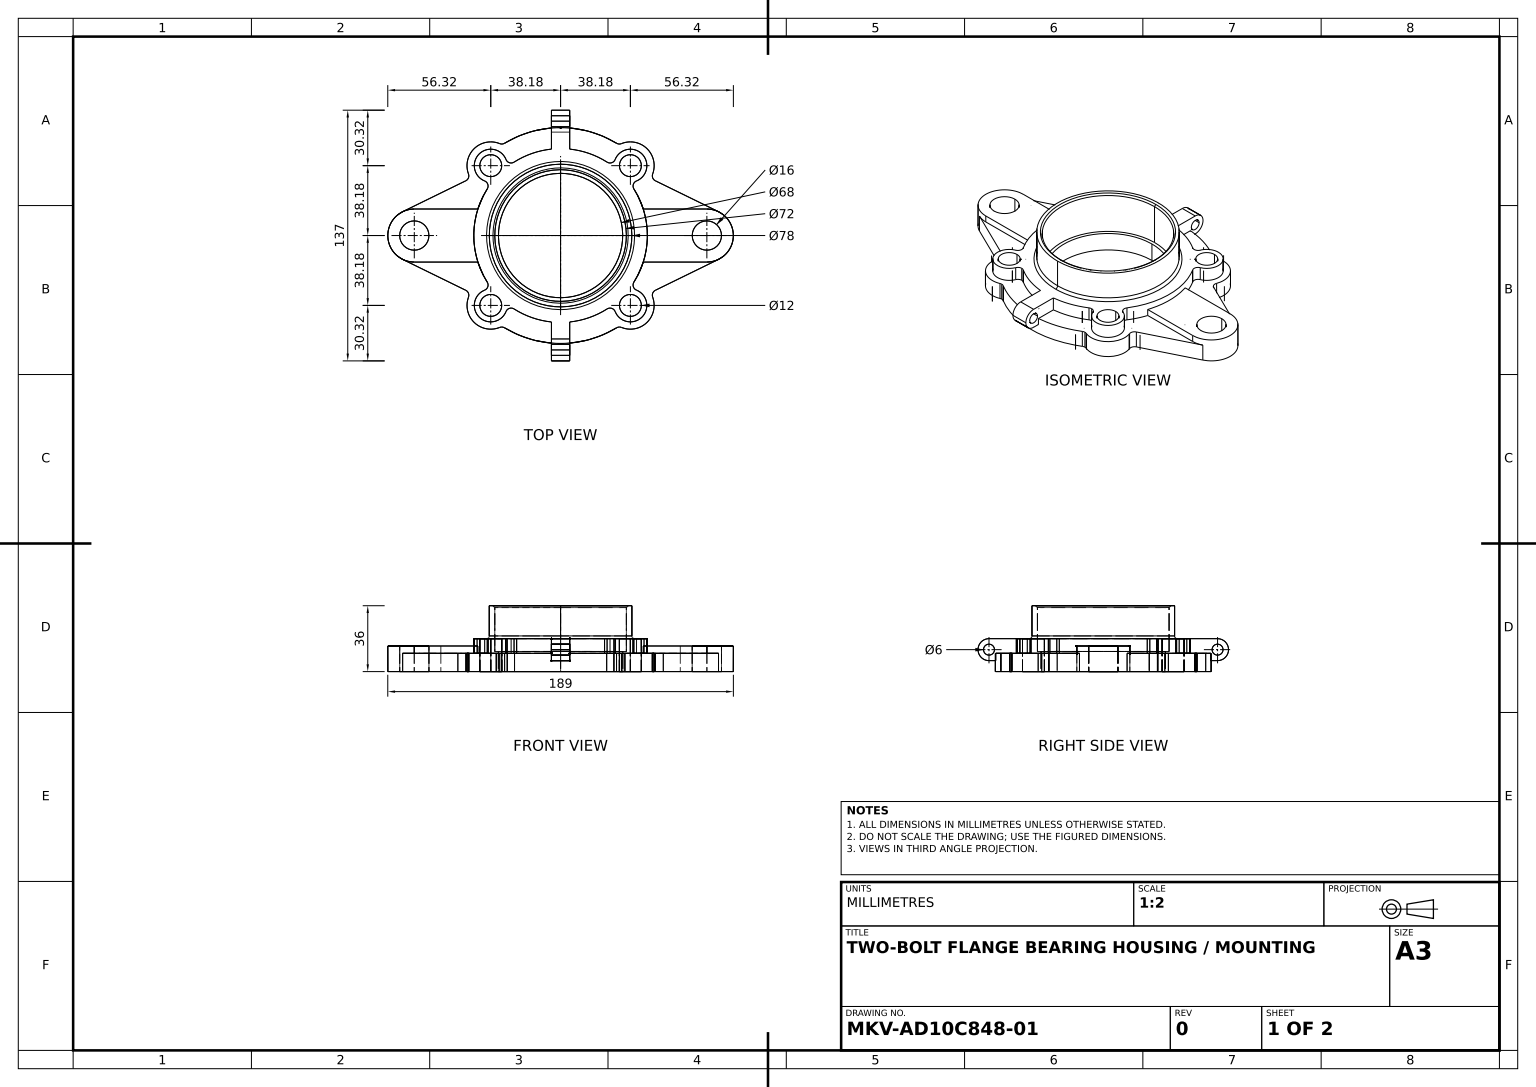
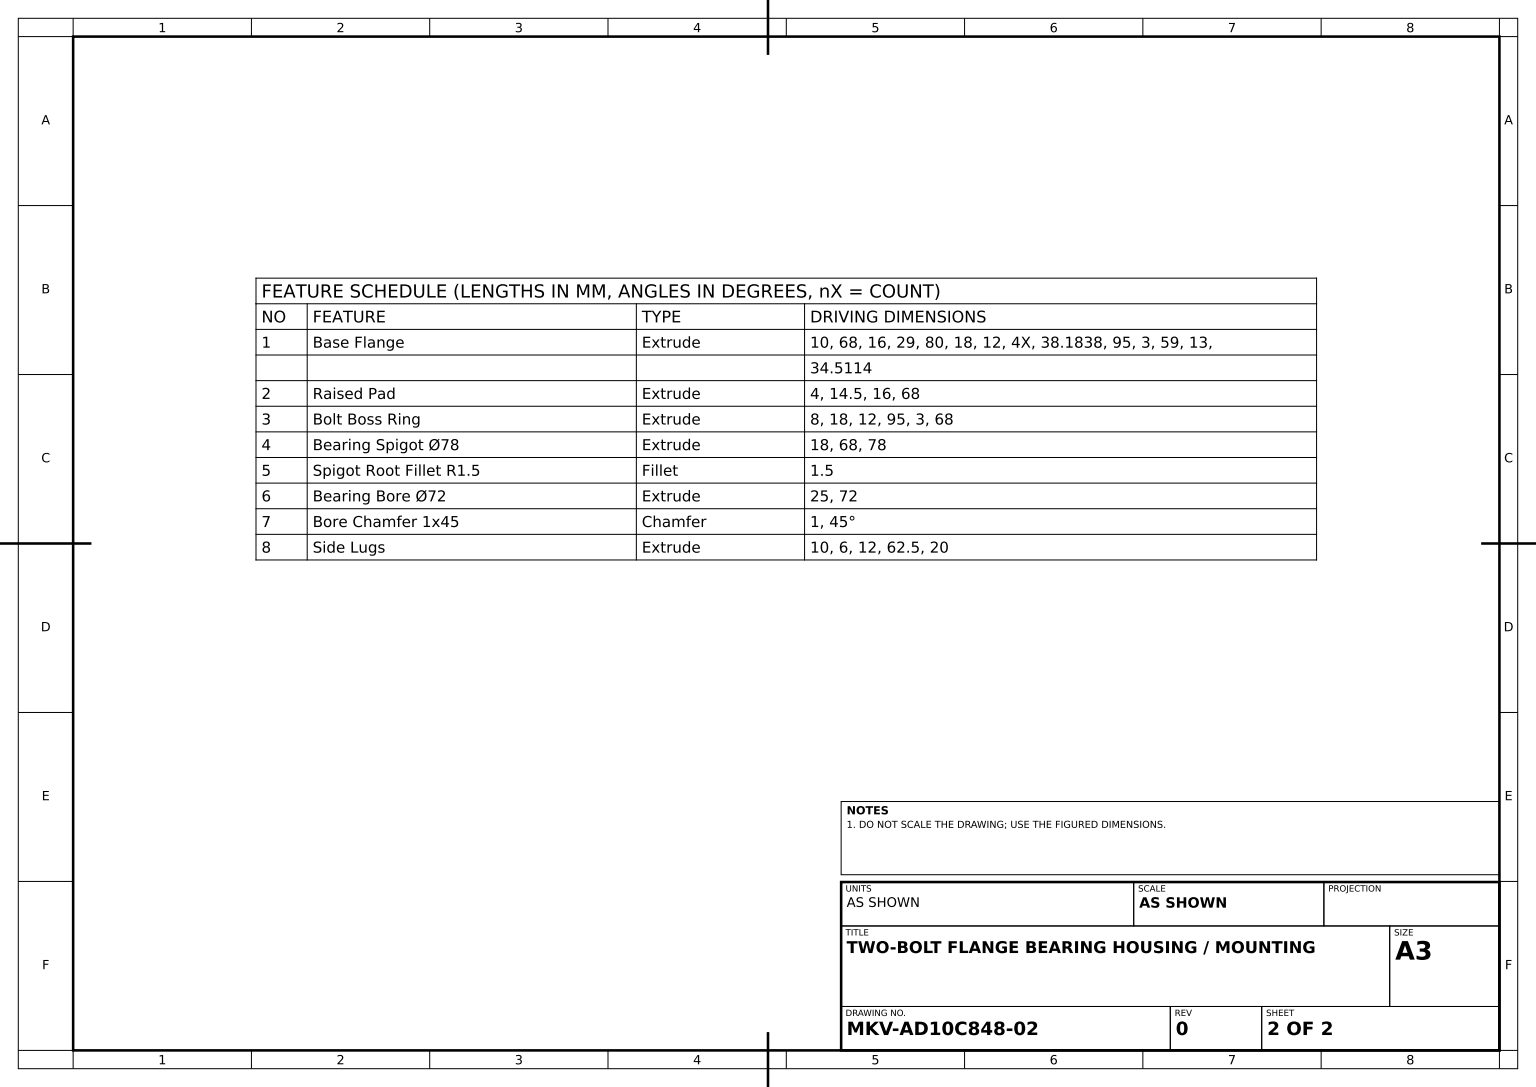
from build123d import *

# Parameters (mm, degrees)
BASE_FLANGE_SKETCH_R      = 8
BASE_FLANGE_SKETCH_R_2    = 34
BASE_FLANGE_SKETCH_R_3    = 6
BASE_FLANGE_DEPTH         = 10
RAISED_PAD_SKETCH_R       = 8
RAISED_PAD_DEPTH          = 4
BOLT_BOSS_RING_SKETCH_R   = 6
BOLT_BOSS_RING_SKETCH_R_2 = 34
BOLT_BOSS_RING_DEPTH      = 8
BEARING_SPIGOT_SKETCH_R   = 39
BEARING_SPIGOT_SKETCH_R_2 = 34
BEARING_SPIGOT_78_DEPTH   = 18
SPIGOT_ROOT_FILLET_R1_5_R = 1.5
BEARING_BORE_SKETCH_R     = 36
BEARING_BORE_72_DEPTH     = 25
BORE_CHAMFER_1X45_SIZE    = 1
SIDE_LUGS_SKETCH_R        = 3
SIDE_LUGS_DEPTH           = 5


with BuildPart() as part:
    # Base Flange Sketch → Base Flange (new body)
    # profile 1 of 5: a face of its own
    with BuildSketch(Plane(origin=(0, 0, 0), x_dir=(1, 0, 0), z_dir=(0, 1, 0))):
        with BuildLine():
            ThreePointArc((-80, 14.5), (-83.270528886, 14.126345628), (-86.372499507, 13.024640112))
            ThreePointArc((-86.372499507, 13.024640112), (-94.5, 0), (-86.372499507, -13.024640112))
            ThreePointArc((-86.372499507, -13.024640112), (-83.270528886, -14.126345628), (-80, -14.5))
            Line((-80, -14.5), (-45.232731512, -14.5))
            ThreePointArc((-45.232731512, -14.5), (-47.5, 0), (-45.232731512, 14.5))
            Line((-45.232731512, 14.5), (-80, 14.5))
        make_face()
        with Locations(Location((-80, 0, 0), (0, 0, 270))):
            Circle(BASE_FLANGE_SKETCH_R, mode=Mode.SUBTRACT)
    # profile 2 of 5: a face of its own
    with BuildSketch(Plane(origin=(0, 0, 0), x_dir=(1, 0, 0), z_dir=(0, 1, 0))):
        with BuildLine():
            ThreePointArc((-80, -14.5), (-83.270528886, -14.126345628), (-86.372499507, -13.024640112))
            Line((-86.372499507, -13.024640112), (-51.861087106, -29.909863551))
            ThreePointArc((-51.861087106, -29.909863551), (-50.393315143, -31.492421844), (-50.367828575, -33.65070721))
            ThreePointArc((-50.367828575, -33.65070721), (-47.238206932, -47.512061995), (-33.289777567, -50.227390033))
            ThreePointArc((-33.289777567, -50.227390033), (-31.921585171, -50.016208018), (-30.604247405, -50.44184811))
            ThreePointArc((-30.604247405, -50.44184811), (0, -59), (30.604247405, -50.44184811))
            ThreePointArc((30.604247405, -50.44184811), (31.921585171, -50.016208018), (33.289777567, -50.227390033))
            ThreePointArc((33.289777567, -50.227390033), (47.238206932, -47.512061995), (50.367828575, -33.65070721))
            ThreePointArc((50.367828575, -33.65070721), (50.393315143, -31.492421844), (51.861087106, -29.909863551))
            Line((51.861087106, -29.909863551), (86.372499507, -13.024640112))
            ThreePointArc((86.372499507, -13.024640112), (83.270528886, -14.126345628), (80, -14.5))
            Line((80, -14.5), (45.232731512, -14.5))
            ThreePointArc((45.232731512, -14.5), (43.022471721, -20.132484374), (40.114125183, -25.438297128))
            ThreePointArc((40.114125183, -25.438297128), (39.792711515, -27.966518872), (41.531678205, -29.829636361))
            ThreePointArc((41.531678205, -29.829636361), (44.547727215, -44.547727215), (29.829636361, -41.531678205))
            ThreePointArc((29.829636361, -41.531678205), (27.966518872, -39.792711515), (25.438297128, -40.114125183))
            ThreePointArc((25.438297128, -40.114125183), (0, -47.5), (-25.438297128, -40.114125183))
            ThreePointArc((-25.438297128, -40.114125183), (-27.966518872, -39.792711515), (-29.829636361, -41.531678205))
            ThreePointArc((-29.829636361, -41.531678205), (-44.547727215, -44.547727215), (-41.531678205, -29.829636361))
            ThreePointArc((-41.531678205, -29.829636361), (-39.792711515, -27.966518872), (-40.114125183, -25.438297128))
            ThreePointArc((-40.114125183, -25.438297128), (-43.022471721, -20.132484374), (-45.232731512, -14.5))
            Line((-45.232731512, -14.5), (-80, -14.5))
        make_face()
    # profile 3 of 5: a face of its own
    with BuildSketch(Plane(origin=(0, 0, 0), x_dir=(1, 0, 0), z_dir=(0, 1, 0))):
        with BuildLine():
            Line((-51.861087106, 29.909863551), (-86.372499507, 13.024640112))
            ThreePointArc((-86.372499507, 13.024640112), (-83.270528886, 14.126345628), (-80, 14.5))
            Line((-80, 14.5), (-45.232731512, 14.5))
            ThreePointArc((-45.232731512, 14.5), (-43.022471721, 20.132484374), (-40.114125183, 25.438297128))
            ThreePointArc((-40.114125183, 25.438297128), (-39.792711515, 27.966518872), (-41.531678205, 29.829636361))
            ThreePointArc((-41.531678205, 29.829636361), (-44.547727215, 44.547727215), (-29.829636361, 41.531678205))
            ThreePointArc((-29.829636361, 41.531678205), (-27.966518872, 39.792711515), (-25.438297128, 40.114125183))
            ThreePointArc((-25.438297128, 40.114125183), (0, 47.5), (25.438297128, 40.114125183))
            ThreePointArc((25.438297128, 40.114125183), (27.966518872, 39.792711515), (29.829636361, 41.531678205))
            ThreePointArc((29.829636361, 41.531678205), (44.547727215, 44.547727215), (41.531678205, 29.829636361))
            ThreePointArc((41.531678205, 29.829636361), (39.792711515, 27.966518872), (40.114125183, 25.438297128))
            ThreePointArc((40.114125183, 25.438297128), (43.022471721, 20.132484374), (45.232731512, 14.5))
            Line((45.232731512, 14.5), (80, 14.5))
            ThreePointArc((80, 14.5), (83.270528886, 14.126345628), (86.372499507, 13.024640112))
            Line((86.372499507, 13.024640112), (51.861087106, 29.909863551))
            ThreePointArc((51.861087106, 29.909863551), (50.393315143, 31.492421844), (50.367828575, 33.65070721))
            ThreePointArc((50.367828575, 33.65070721), (47.238206932, 47.512061995), (33.289777567, 50.227390033))
            ThreePointArc((33.289777567, 50.227390033), (31.921585171, 50.016208018), (30.604247405, 50.44184811))
            ThreePointArc((30.604247405, 50.44184811), (0, 59), (-30.604247405, 50.44184811))
            ThreePointArc((-30.604247405, 50.44184811), (-31.921585171, 50.016208018), (-33.289777567, 50.227390033))
            ThreePointArc((-33.289777567, 50.227390033), (-47.238206932, 47.512061995), (-50.367828575, 33.65070721))
            ThreePointArc((-50.367828575, 33.65070721), (-50.393315143, 31.492421844), (-51.861087106, 29.909863551))
        make_face()
    # profile 4 of 5: a face of its own
    with BuildSketch(Plane(origin=(0, 0, 0), x_dir=(1, 0, 0), z_dir=(0, 1, 0))):
        with BuildLine():
            ThreePointArc((86.372499507, -13.024640112), (94.5, 0), (86.372499507, 13.024640112))
            ThreePointArc((86.372499507, 13.024640112), (83.270528886, 14.126345628), (80, 14.5))
            Line((80, 14.5), (45.232731512, 14.5))
            ThreePointArc((45.232731512, 14.5), (47.5, 0), (45.232731512, -14.5))
            Line((45.232731512, -14.5), (80, -14.5))
            ThreePointArc((80, -14.5), (83.270528886, -14.126345628), (86.372499507, -13.024640112))
        make_face()
        with Locations(Location((80, 0, 0), (0, 0, 270))):
            Circle(BASE_FLANGE_SKETCH_R, mode=Mode.SUBTRACT)
    # profile 5 of 5: a face of its own
    with BuildSketch(Plane(origin=(0, 0, 0), x_dir=(1, 0, 0), z_dir=(0, 1, 0))):
        with BuildLine():
            ThreePointArc((-41.531678205, -29.829636361), (-44.547727215, -44.547727215), (-29.829636361, -41.531678205))
            ThreePointArc((-29.829636361, -41.531678205), (-27.966518872, -39.792711515), (-25.438297128, -40.114125183))
            ThreePointArc((-25.438297128, -40.114125183), (0, -47.5), (25.438297128, -40.114125183))
            ThreePointArc((25.438297128, -40.114125183), (27.966518872, -39.792711515), (29.829636361, -41.531678205))
            ThreePointArc((29.829636361, -41.531678205), (44.547727215, -44.547727215), (41.531678205, -29.829636361))
            ThreePointArc((41.531678205, -29.829636361), (39.792711515, -27.966518872), (40.114125183, -25.438297128))
            ThreePointArc((40.114125183, -25.438297128), (47.5, 0), (40.114125183, 25.438297128))
            ThreePointArc((40.114125183, 25.438297128), (39.792711515, 27.966518872), (41.531678205, 29.829636361))
            ThreePointArc((41.531678205, 29.829636361), (44.547727215, 44.547727215), (29.829636361, 41.531678205))
            ThreePointArc((29.829636361, 41.531678205), (27.966518872, 39.792711515), (25.438297128, 40.114125183))
            ThreePointArc((25.438297128, 40.114125183), (0, 47.5), (-25.438297128, 40.114125183))
            ThreePointArc((-25.438297128, 40.114125183), (-27.966518872, 39.792711515), (-29.829636361, 41.531678205))
            ThreePointArc((-29.829636361, 41.531678205), (-44.547727215, 44.547727215), (-41.531678205, 29.829636361))
            ThreePointArc((-41.531678205, 29.829636361), (-39.792711515, 27.966518872), (-40.114125183, 25.438297128))
            ThreePointArc((-40.114125183, 25.438297128), (-47.5, 0), (-40.114125183, -25.438297128))
            ThreePointArc((-40.114125183, -25.438297128), (-39.792711515, -27.966518872), (-41.531678205, -29.829636361))
        make_face()
        with Locations(Location((0, 0, 0), (0, 0, 270))):
            Circle(BASE_FLANGE_SKETCH_R_2, mode=Mode.SUBTRACT)
        with Locations(Location((-38.183766184, 38.183766184, 0), (0, 0, 270))):
            Circle(BASE_FLANGE_SKETCH_R_3, mode=Mode.SUBTRACT)
        with Locations(Location((38.183766184, 38.183766184, 0), (0, 0, 270))):
            Circle(BASE_FLANGE_SKETCH_R_3, mode=Mode.SUBTRACT)
        with Locations(Location((38.183766184, -38.183766184, 0), (0, 0, 270))):
            Circle(BASE_FLANGE_SKETCH_R_3, mode=Mode.SUBTRACT)
        with Locations(Location((-38.183766184, -38.183766184, 0), (0, 0, 270))):
            Circle(BASE_FLANGE_SKETCH_R_3, mode=Mode.SUBTRACT)
    extrude(amount=BASE_FLANGE_DEPTH)

    # Raised Pad Sketch → Raised Pad (add)
    # profile 1 of 2: a face of its own
    with BuildSketch(Plane(origin=(0, 10, 0), x_dir=(1, 0, 0), z_dir=(0, 1, 0))):
        with BuildLine():
            Line((-80, 14.5), (-30.753048629, 14.5))
            ThreePointArc((-30.753048629, 14.5), (-34, 0), (-30.753048629, -14.5))
            Line((-30.753048629, -14.5), (-80, -14.5))
            ThreePointArc((-80, -14.5), (-94.5, 0), (-80, 14.5))
        make_face()
        with Locations(Location((-80, 0, 0), (0, 0, 270))):
            Circle(RAISED_PAD_SKETCH_R, mode=Mode.SUBTRACT)
    # profile 2 of 2: a face of its own
    with BuildSketch(Plane(origin=(0, 10, 0), x_dir=(1, 0, 0), z_dir=(0, 1, 0))):
        with BuildLine():
            Line((80, -14.5), (30.753048629, -14.5))
            ThreePointArc((30.753048629, -14.5), (34, 0), (30.753048629, 14.5))
            Line((30.753048629, 14.5), (80, 14.5))
            ThreePointArc((80, 14.5), (94.5, 0), (80, -14.5))
        make_face()
        with Locations(Location((80, 0, 0), (0, 0, 270))):
            Circle(RAISED_PAD_SKETCH_R, mode=Mode.SUBTRACT)
    extrude(amount=RAISED_PAD_DEPTH)

    # Bolt Boss Ring Sketch → Bolt Boss Ring (add)
    with BuildSketch(Plane(origin=(0, 10, 0), x_dir=(1, 0, 0), z_dir=(0, 1, 0))):
        with BuildLine():
            ThreePointArc((-29.829636361, 41.531678205), (-44.547727215, 44.547727215), (-41.531678205, 29.829636361))
            ThreePointArc((-41.531678205, 29.829636361), (-39.792711515, 27.966518872), (-40.114125183, 25.438297128))
            ThreePointArc((-40.114125183, 25.438297128), (-47.5, 0), (-40.114125183, -25.438297128))
            ThreePointArc((-40.114125183, -25.438297128), (-39.792711515, -27.966518872), (-41.531678205, -29.829636361))
            ThreePointArc((-41.531678205, -29.829636361), (-44.547727215, -44.547727215), (-29.829636361, -41.531678205))
            ThreePointArc((-29.829636361, -41.531678205), (-27.966518872, -39.792711515), (-25.438297128, -40.114125183))
            ThreePointArc((-25.438297128, -40.114125183), (0, -47.5), (25.438297128, -40.114125183))
            ThreePointArc((25.438297128, -40.114125183), (27.966518872, -39.792711515), (29.829636361, -41.531678205))
            ThreePointArc((29.829636361, -41.531678205), (44.547727215, -44.547727215), (41.531678205, -29.829636361))
            ThreePointArc((41.531678205, -29.829636361), (39.792711515, -27.966518872), (40.114125183, -25.438297128))
            ThreePointArc((40.114125183, -25.438297128), (47.5, 0), (40.114125183, 25.438297128))
            ThreePointArc((40.114125183, 25.438297128), (39.792711515, 27.966518872), (41.531678205, 29.829636361))
            ThreePointArc((41.531678205, 29.829636361), (44.547727215, 44.547727215), (29.829636361, 41.531678205))
            ThreePointArc((29.829636361, 41.531678205), (27.966518872, 39.792711515), (25.438297128, 40.114125183))
            ThreePointArc((25.438297128, 40.114125183), (0, 47.5), (-25.438297128, 40.114125183))
            ThreePointArc((-25.438297128, 40.114125183), (-27.966518872, 39.792711515), (-29.829636361, 41.531678205))
        make_face()
        with Locations(Location((-38.183766184, 38.183766184, 0), (0, 0, 270))):
            Circle(BOLT_BOSS_RING_SKETCH_R, mode=Mode.SUBTRACT)
        with Locations(Location((38.183766184, 38.183766184, 0), (0, 0, 270))):
            Circle(BOLT_BOSS_RING_SKETCH_R, mode=Mode.SUBTRACT)
        with Locations(Location((38.183766184, -38.183766184, 0), (0, 0, 270))):
            Circle(BOLT_BOSS_RING_SKETCH_R, mode=Mode.SUBTRACT)
        with Locations(Location((-38.183766184, -38.183766184, 0), (0, 0, 270))):
            Circle(BOLT_BOSS_RING_SKETCH_R, mode=Mode.SUBTRACT)
        with Locations(Location((0, 0, 0), (0, 0, 270))):
            Circle(BOLT_BOSS_RING_SKETCH_R_2, mode=Mode.SUBTRACT)
    extrude(amount=BOLT_BOSS_RING_DEPTH)

    # Bearing Spigot Sketch → Bearing Spigot Ø78 (add)
    with BuildSketch(Plane(origin=(0, 18, 0), x_dir=(1, 0, 0), z_dir=(0, 1, 0))):
        with Locations(Location((0, 0, 0), (0, 0, 270))):
            Circle(BEARING_SPIGOT_SKETCH_R)
        with Locations(Location((0, 0, 0), (0, 0, 270))):
            Circle(BEARING_SPIGOT_SKETCH_R_2, mode=Mode.SUBTRACT)
    extrude(amount=BEARING_SPIGOT_78_DEPTH)

    # Spigot Root Fillet R1.5
    spigot_root_fillet_r1_5_edges = [part.edges().sort_by_distance(p)[0] for p in [
        (0, 18, -39),
    ]]
    fillet(spigot_root_fillet_r1_5_edges, radius=SPIGOT_ROOT_FILLET_R1_5_R)

    # Bearing Bore Sketch → Bearing Bore Ø72 (cut)
    with BuildSketch(Plane(origin=(0, 36, 0), x_dir=(1, 0, 0), z_dir=(0, 1, 0))):
        with Locations(Location((0, 0, 0), (0, 0, 270))):
            Circle(BEARING_BORE_SKETCH_R)
    extrude(amount=-BEARING_BORE_72_DEPTH, mode=Mode.SUBTRACT)

    # Bore Chamfer 1x45
    bore_chamfer_1x45_edges = [part.edges().sort_by_distance(p)[0] for p in [
        (0, 36, -36),
    ]]
    chamfer(bore_chamfer_1x45_edges, length=BORE_CHAMFER_1X45_SIZE)

    # Side Lugs Sketch → Side Lugs (add, symmetric)
    # profile 1 of 2: a face of its own
    with BuildSketch(Plane(origin=(0, 0, 0), x_dir=(0, 0, -1), z_dir=(1, 0, 0))):
        with BuildLine():
            Line((-62.5, 18), (-42.5, 18))
            Line((-42.5, 18), (-42.5, 6))
            Line((-42.5, 6), (-62.5, 6))
            ThreePointArc((-62.5, 6), (-68.5, 12), (-62.5, 18))
        make_face()
        with Locations((-62.5, 12)):
            Circle(SIDE_LUGS_SKETCH_R, mode=Mode.SUBTRACT)
    # profile 2 of 2: a face of its own
    with BuildSketch(Plane(origin=(0, 0, 0), x_dir=(0, 0, -1), z_dir=(1, 0, 0))):
        with BuildLine():
            Line((62.5, 18), (42.5, 18))
            Line((42.5, 18), (42.5, 6))
            Line((42.5, 6), (62.5, 6))
            ThreePointArc((62.5, 6), (68.5, 12), (62.5, 18))
        make_face()
        with Locations((62.5, 12)):
            Circle(SIDE_LUGS_SKETCH_R, mode=Mode.SUBTRACT)
    extrude(amount=SIDE_LUGS_DEPTH, both=True)


solid = part.part
